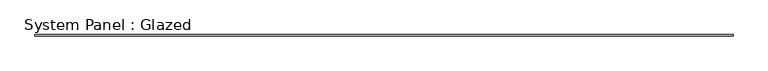
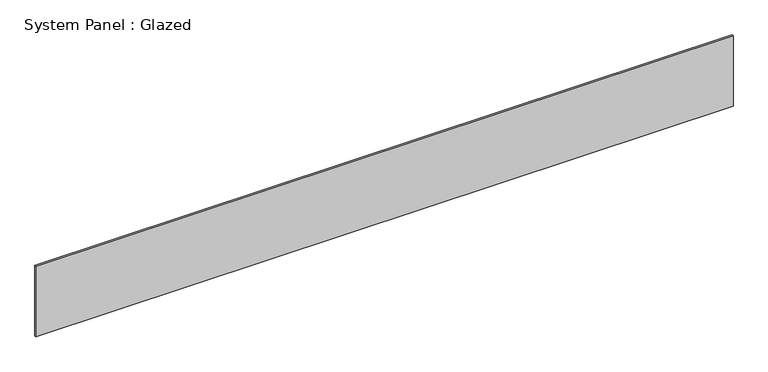
"""IFC4 building model written with IfcOpenShell, lengths in millimetres: plate geometry, System Panel : Glazed."""

from ifc_helpers import new_model, si_unit, origin, origin_with_axes, place, context, project, spatial, polyline, outline, extrude, source, transform, mapped, element, save


def system_panel_glazed_53b9e4d0(model_context):
    return source(origin(), model_context, "Body", "SweptSolid", [
        extrude(outline(polyline([(6834.910375, 19.05), (-6834.910375, 19.05), (-6834.910375, 44.45), (6834.910375, 44.45), (6834.910375, 19.05)])), origin_with_axes(), (0.0, 0.0, 1.0), 1460.5),
    ])


if __name__ == "__main__":
    model = new_model("IFC4")
    model_context = context("Model", 3, world=origin())
    ifc_project = project(units=[si_unit("LENGTHUNIT", "METRE", prefix="MILLI")], contexts=[model_context])
    site = spatial("IfcSite", under=ifc_project)
    building = spatial("IfcBuilding", under=site)
    placement = place(None, origin())
    system_panel_glazed_shape = system_panel_glazed_53b9e4d0(model_context)
    element("IfcPlate", 1, ObjectType="System Panel : Glazed", at=placement, inside=building, context=model_context, shape_type="MappedRepresentation", body=[
        mapped(system_panel_glazed_shape, transform((0.0, 0.0, 0.0), x_axis=(1.0, 0.0, 0.0), y_axis=(0.0, 1.0, 0.0), z_axis=(0.0, 0.0, 1.0))),
    ])
    save(model, "model.ifc")

# Revit data of these elements
# Type "System Panel : Glazed"
#   Construction Type Id = "GSP4R"
#   Analytic Construction = "1/8 in Pilkington single glazing"
#   Visual Light Transmittance = 0.9
#   Solar Heat Gain Coefficient = 0.86
#   Heat Transfer Coefficient (U) = 1.18115 BTU/(h·ft²·°F)
# Element 1 (IfcPlate, "System Panel : Glazed")
#   Materials on its faces: "Glass"
# Materials
#   "Glass": class "Glass", colour RGB 0 128 192, transparency 0.75, Description = "Soda Lime Glass", Cost = 0
